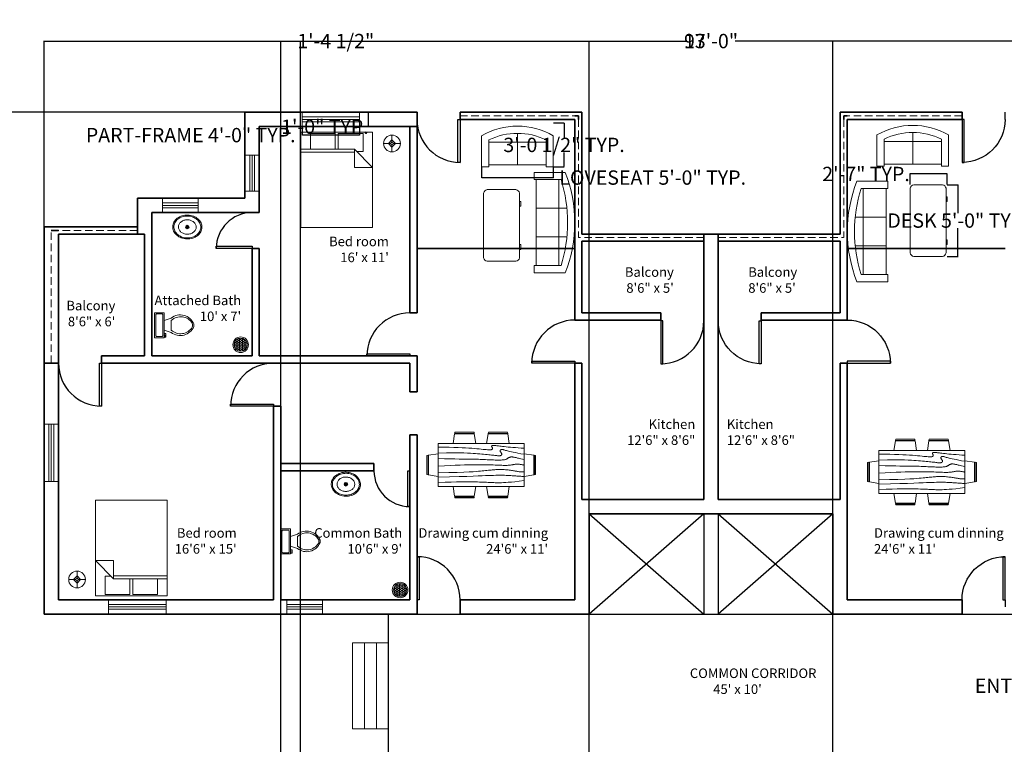
# Model space of a CAD drawing. Units: inches. Extents: x 2450 to 4494, y 1482 to 2597.
# Tile 6 of 7: x 3238 to 4062, y 1990 to 2597. Entities that reach past the tile are written whole.
import ezdxf

# ---------------------------------------------------------------- set-up
doc = ezdxf.new("R2010")
doc.units = ezdxf.units.IN
doc.header["$LTSCALE"] = 5
doc.header["$MEASUREMENT"] = 0
doc.linetypes.add('HIDDEN', pattern=[0.375, 0.25, -0.125])
for name, color, linetype, lineweight in [('A-ANNO-DIMS', 2, 'Continuous', 18), ('A-AREA-IDEN', 7, 'Continuous', 18), ('A-DOOR', 4, 'Continuous', 25), ('A-FLOR-EDGE', 7, 'Continuous', 25), ('A-FLOR-EVTR', 6, 'Continuous', 25), ('A-FLOR-FIXT', 9, 'Continuous', 18), ('A-FLOR-STRS', 7, 'Continuous', 18), ('A-FURN', 8, 'Continuous', 18), ('A-GLAZ', 4, 'Continuous', 18), ('A-WALL', 7, 'Continuous', 35), ('A-WALL-HIDN', 7, 'HIDDEN', 18)]:
    doc.layers.add(name, color=color, linetype=linetype, lineweight=lineweight)
doc.styles.get("Standard").update_dxf_attribs({"font": 'arial.ttf'})
doc.dimstyles.get("Standard").update_dxf_attribs({"dimtxt": 12, "dimasz": 0.18, "dimexe": 0.18, "dimexo": 0.0625, "dimgap": 0.09, "dimtad": 0, "dimtih": 1, "dimtoh": 1, "dimdec": 0, "dimzin": 0, "dimdsep": 46, "dimlunit": 3, "dimtxsty": 'Standard', "dimcen": 0.09, "dimadec": 0, "dimazin": 0, "dimtfac": 1, "dimtdec": 0, "dimtofl": 0, "dimtmove": 0, "dimatfit": 3, "dimfxl": 1, "dimtolj": 1, "dimtzin": 0, "dimarcsym": 0})

# ---------------------------------------------------------------- blocks, each defined once
blk = doc.blocks.new('*U4')
for p, q in [((-36, 0), (-36, -6)), ((0, 0), (0, -6))]:
    blk.add_line(p, q)
blk.add_lwpolyline([(0, 0), (0, 36), (-1.75, 36), (-1.75, 0)], close=True)
blk.add_arc((0, 0), 36, 90, 180)
blk = doc.blocks.new('*U2')
for p, q in [((0, 0), (0, -6)), ((36, 0), (36, -6))]:
    blk.add_line(p, q)
blk.add_lwpolyline([(0, 0), (0, 36), (1.75, 36), (1.75, 0)], close=True)
blk.add_arc((0, 0), 36, 0, 90)
blk = doc.blocks.new('*U5')
for p, q in [((-36, 0), (-36, 6)), ((0, 0), (0, 6))]:
    blk.add_line(p, q)
blk.add_lwpolyline([(0, 0), (0, -36), (-1.75, -36), (-1.75, 0)], close=True)
blk.add_arc((0, 0), 36, 180, 270)
blk = doc.blocks.new('*U3')
for p, q in [((0, 0), (0, -6)), ((30, 0), (30, -6))]:
    blk.add_line(p, q)
blk.add_lwpolyline([(0, 0), (0, 30), (1.75, 30), (1.75, 0)], close=True)
blk.add_arc((0, 0), 30, 0, 90)
blk = doc.blocks.new('Bed - Queen')
for p, q in [((0, -80.00003), (0, 0)), ((0, 0), (59.99999, 0)), ((59.99999, 0), (59.99999, -80.00003)), ((7.99999, -1.2), (28.79998, -1.2)), ((7.99999, -14.4), (7.99999, -1.2)), ((28.79998, -1.2), (28.79998, -14.4)), ((31.19999, -1.2), (51.99999, -1.2)), ((31.19999, -14.4), (31.19999, -1.2)), ((51.99999, -1.2), (51.99999, -16.4)), ((0, -14.4), (44.8, -14.4)), ((59.99999, -29.6), (44.8, -14.4)), ((44.8, -14.4), (44.8, -29.6)), ((51.99999, -16.4), (46.79936, -16.4)), ((44.8, -16.8), (0, -16.8)), ((44.8, -29.6), (59.99999, -29.6)), ((59.99999, -80.00003), (0, -80.00003))]:
    blk.add_line(p, q)
blk = doc.blocks.new('Lamp - Table')
for p, q in [((-1, 0), (-7, 0)), ((0, 3), (-3, 0)), ((-3, 0), (0, -3)), ((0, 7), (0, 1)), ((3, 0), (0, 3)), ((0, -3), (3, 0)), ((1, 0), (7, 0)), ((0, -1), (0, -7))]:
    blk.add_line(p, q)
for radius in [7, 1]:
    blk.add_circle((0, 0), radius)
blk = doc.blocks.new('Toilet - top')
for p, q in [((-8, -8.5), (-8, -8)), ((-7, -8), (-7, -9.5)), ((-4, -8), (-6, -14)), ((4, -8), (6, -14)), ((9.5, -6), (9.5, -2)), ((-10, -8.5), (-8, -8.5)), ((-10, -9.5), (-10, -8.5)), ((-7, -9.5), (-10, -9.5)), ((4, -14), (-4, -14))]:
    blk.add_line(p, q)
blk.add_lwpolyline([(10.5, -8), (10.5, 0), (-10.5, 0), (-10.5, -8)], close=True)
for points in [[(-9.5, -2), (-9.5, -6)], [(8.5, -1), (-8.5, -1)], [(-8.5, -7), (8.5, -7)]]:
    blk.add_lwpolyline(points)
for centre, radius, start, end in [((-8.62, -1.88), 0.884, 81.8699, 188.1301), ((-8.62, -6.12), 0.884, 171.8699, 278.1301), ((8.62, -1.88), 0.884, 351.8699, 98.1301), ((8.62, -6.12), 0.884, 261.8699, 8.1301), ((3.52, -21.58), 12.17, 141.46911, 247.97143), ((4.2, -21.82), 11.33, 136.36773, 238.94682), ((-3.52, -21.58), 12.17, 292.02843, 38.53071), ((-4.2, -21.82), 11.33, 301.05301, 43.63209), ((0, -27.88), 4, 245.73182, 294.26817), ((0, -29), 4, 254.86053, 285.13947)]:
    blk.add_arc(centre, radius, start, end)
blk = doc.blocks.new('Sink - Oval top')
for p, q in [((-1, 0), (1, 0)), ((0, 1), (0, -1))]:
    blk.add_line(p, q)
for points in [[(-12.23, 0.39, 0.117634), (-11.46, -3.36, 0.104469), (-8.88, -6.8, 0.090016), (-5.08, -9.07, 0.08192), (-0.32, -10.02, 0.08192), (4.49, -9.38, 0.090016), (8.42, -7.36, 0.104469), (11.22, -4.09, 0.117634), (12.23, -0.39, 0.117634), (11.46, 3.36, 0.104469), (8.88, 6.8, 0.090016), (5.08, 9.07, 0.08192), (0.32, 10.02, 0.08192), (-4.49, 9.38, 0.090016), (-8.42, 7.36, 0.104469), (-11.22, 4.09, 0.117634)], [(-11.29, 0.16, 0.118622), (-10.52, -3.25, 0.104678), (-8.07, -6.36, 0.089562), (-4.54, -8.37, 0.081185), (-0.13, -9.15, 0.081185), (4.3, -8.49, 0.089562), (7.89, -6.58, 0.104678), (10.42, -3.55, 0.118622), (11.29, -0.16, 0.118622), (10.52, 3.25, 0.104678), (8.07, 6.36, 0.089562), (4.54, 8.37, 0.081185), (0.13, 9.15, 0.081185), (-4.3, 8.49, 0.089562), (-7.89, 6.58, 0.104678), (-10.42, 3.55, 0.118622)], [(-7.42, 0.08, 0.118283), (-6.91, -2.17, 0.104607), (-5.29, -4.21, 0.089718), (-2.97, -5.53, 0.081436), (-0.07, -6.04, 0.081436), (2.84, -5.59, 0.089718), (5.2, -4.33, 0.104607), (6.86, -2.32, 0.118283), (7.42, -0.08, 0.118283), (6.91, 2.17, 0.104607), (5.29, 4.21, 0.089718), (2.97, 5.53, 0.081436), (0.07, 6.04, 0.081436), (-2.84, 5.59, 0.089718), (-5.2, 4.33, 0.104607), (-6.86, 2.32, 0.118283)]]:
    blk.add_lwpolyline(points, format="xyb", close=True)
for radius in [1.5, 1]:
    blk.add_circle((0, 0), radius)
blk = doc.blocks.new('Dining Set - 36 x 72 in.')
for p, q in [((-22.2343, 26.00059), (-23.4847, 17.99762)), ((-22.2304, 26), (-5.7608, 26)), ((-22, 27.5), (-22.1562, 26.50042)), ((-5.8416, 26.5), (-22.1534, 26.5)), ((-22, 27.5), (-6, 27.5)), ((-5.8437, 26.49966), (-6, 27.5)), ((-4.5152, 17.99762), (-5.7655, 25.99926)), ((5.7657, 26.00059), (4.5153, 17.99762)), ((5.7696, 26), (22.2392, 26)), ((6, 27.5), (5.8438, 26.50042)), ((22.1584, 26.5), (5.8466, 26.5)), ((6, 27.5), (22, 27.5)), ((22.1563, 26.49966), (22, 27.5)), ((23.4848, 17.99762), (22.2345, 25.99926)), ((36, 18), (-36, 18)), ((-36, 18), (-36, -18)), ((36, -18), (36, 18)), ((-44.0006, 8.23428), (-35.9976, 9.48474)), ((44.0006, 8.23428), (35.9976, 9.48474)), ((-45.5, 8), (-44.5004, 8.15617)), ((-45.5, 8), (-45.5, -8)), ((-44.5, -8.15843), (-44.5, 8.15338)), ((-44, 8.23041), (-44, -8.23915)), ((44, 8.23041), (44, -8.23915)), ((44.5, -8.15843), (44.5, 8.15338)), ((45.5, 8), (44.5005, 8.15617)), ((45.5, 8), (45.5, -8)), ((-44.4997, -8.15631), (-45.5, -8)), ((-35.9976, -9.48476), (-43.9993, -8.2345)), ((35.9976, -9.48476), (43.9993, -8.2345)), ((44.4997, -8.15631), (45.5, -8)), ((-36, -18), (36, -18)), ((-22.2343, -26.0006), (-23.4847, -17.99762)), ((-4.5152, -17.99762), (-5.7655, -25.99928)), ((5.7657, -26.0006), (4.5153, -17.99762)), ((23.4848, -17.99762), (22.2345, -25.99928)), ((-22.2304, -26), (-5.7608, -26)), ((-22, -27.5), (-22.1562, -26.50044)), ((-5.8416, -26.5), (-22.1534, -26.5)), ((-22, -27.5), (-6, -27.5)), ((-5.8437, -26.49967), (-6, -27.5)), ((5.7696, -26), (22.2392, -26)), ((6, -27.5), (5.8438, -26.50044)), ((22.1584, -26.5), (5.8466, -26.5)), ((6, -27.5), (22, -27.5)), ((22.1563, -26.49967), (22, -27.5))]:
    blk.add_line(p, q)
for points in [[(-36, 15), (-31.1772, 14.97754), (-26.8079, 14.91406), (-22.8538, 14.81543), (-19.276, 14.6875), (-16.0362, 14.53613), (-13.0957, 14.36718), (-10.4159, 14.18652), (-7.9583, 14), (-5.6904, 13.81315), (-3.6035, 13.63021), (-1.6954, 13.45508), (0.0365, 13.29166), (1.5945, 13.14388), (2.9811, 13.01562), (4.1988, 12.9108), (5.25, 12.83333), (6.1393, 12.78613), (6.8802, 12.76823), (7.4883, 12.77767), (7.9792, 12.8125), (8.3685, 12.87077), (8.6719, 12.95052), (8.9049, 13.0498), (9.0833, 13.16666), (9.2205, 13.29899), (9.3216, 13.44401), (9.3895, 13.59879), (9.4271, 13.76041), (9.4373, 13.92594), (9.4232, 14.09245), (9.3875, 14.257), (9.3333, 14.41666), (9.2638, 14.56917), (9.1836, 14.71484), (9.0975, 14.85465), (9.0104, 14.98958), (8.9272, 15.1206), (8.8529, 15.2487), (8.7922, 15.37483), (8.75, 15.5), (8.7305, 15.62467), (8.7344, 15.74739), (8.7617, 15.86621), (8.8125, 15.97916), (8.8867, 16.08431), (8.9844, 16.17968), (9.1055, 16.26334), (9.25, 16.33333), (9.4189, 16.38802), (9.6172, 16.42708), (9.8506, 16.45052), (10.125, 16.45833), (10.4463, 16.45052), (10.8203, 16.42708), (11.2529, 16.38802), (11.75, 16.33333), (12.3184, 16.26318), (12.9694, 16.17838), (13.7151, 16.07991), (14.5677, 15.96875), (15.5395, 15.84586), (16.6426, 15.71224), (17.8893, 15.56884), (19.2917, 15.41666), (20.859, 15.25667), (22.5879, 15.08984), (24.4721, 14.91715), (26.5052, 14.73958), (28.6809, 14.5581), (30.9929, 14.3737), (33.4347, 14.18733), (36, 14)], [(-36, 10), (-28.9766, 10.14274), (-23.1725, 10.20442), (-18.4241, 10.19775), (-14.5677, 10.13541), (-11.4399, 10.03011), (-8.877, 9.89453), (-6.7154, 9.74137), (-4.7917, 9.58333), (-2.9698, 9.43082), (-1.2246, 9.28515), (0.4415, 9.14534), (2.026, 9.01041), (3.5266, 8.87939), (4.9408, 8.7513), (6.266, 8.62516), (7.5, 8.5), (8.6411, 8.37549), (9.6914, 8.2539), (10.6538, 8.13818), (11.5312, 8.03125), (12.3267, 7.93603), (13.043, 7.85547), (13.6831, 7.79248), (14.25, 7.75), (14.7471, 7.7303), (15.1797, 7.73307), (15.5537, 7.75732), (15.875, 7.80208), (16.1494, 7.86637), (16.3828, 7.94922), (16.5811, 8.04964), (16.75, 8.16666), (16.8944, 8.29915), (17.0143, 8.44531), (17.1089, 8.60319), (17.1771, 8.77083), (17.218, 8.94629), (17.2305, 9.1276), (17.2137, 9.31282), (17.1667, 9.5), (17.0895, 9.6875), (16.987, 9.875), (16.8649, 10.0625), (16.7292, 10.25), (16.5856, 10.4375), (16.4401, 10.625), (16.2985, 10.8125), (16.1667, 11), (16.05, 11.18733), (15.9518, 11.3737), (15.8752, 11.5581), (15.8229, 11.73958), (15.798, 11.91715), (15.8034, 12.08984), (15.842, 12.25667), (15.9167, 12.41666), (16.0295, 12.56836), (16.1784, 12.70833), (16.3605, 12.83268), (16.5729, 12.9375), (16.8127, 13.01888), (17.0768, 13.07291), (17.3625, 13.0957), (17.6667, 13.08333), (17.9894, 13.03312), (18.3418, 12.94726), (18.7382, 12.82918), (19.1927, 12.68229), (19.7195, 12.51001), (20.3327, 12.31575), (21.0465, 12.10294), (21.875, 11.875), (22.8357, 11.63354), (23.959, 11.37304), (25.2786, 11.08618), (26.8282, 10.76562), (28.6414, 10.40405), (30.752, 9.99414), (33.1936, 9.52856), (36, 9)], [(-36, 5.5), (-30.7157, 5.3348), (-26.069, 5.20963), (-21.9946, 5.11767), (-18.4271, 5.05208), (-15.3009, 5.00602), (-12.5508, 4.97265), (-10.1112, 4.94515), (-7.9167, 4.91666), (-5.909, 4.88167), (-4.0586, 4.83984), (-2.3429, 4.79215), (-0.7396, 4.73958), (0.7739, 4.6831), (2.22, 4.6237), (3.6213, 4.56233), (5, 4.5), (6.373, 4.43782), (7.7344, 4.3776), (9.0723, 4.32129), (10.375, 4.27083), (11.6309, 4.22819), (12.8281, 4.19531), (13.9551, 4.17415), (15, 4.16666), (15.954, 4.17448), (16.819, 4.19791), (17.6001, 4.23698), (18.3021, 4.29166), (18.9299, 4.36198), (19.4883, 4.44791), (19.9823, 4.54948), (20.4167, 4.66666), (20.7969, 4.79899), (21.1302, 4.94401), (21.4245, 5.09879), (21.6875, 5.26041), (21.9271, 5.42594), (22.1511, 5.59245), (22.3672, 5.757), (22.5834, 5.91666), (22.8065, 6.06868), (23.0404, 6.21093), (23.2879, 6.34147), (23.5521, 6.45833), (23.8358, 6.55957), (24.142, 6.64323), (24.4735, 6.70735), (24.8334, 6.75), (25.2235, 6.76969), (25.642, 6.76692), (26.0858, 6.74267), (26.5521, 6.69791), (27.0379, 6.63362), (27.5404, 6.55078), (28.0565, 6.45036), (28.5834, 6.33333), (29.1242, 6.19987), (29.7071, 6.04687), (30.3661, 5.87044), (31.1354, 5.66666), (32.0493, 5.43164), (33.142, 5.16146), (34.4475, 4.85221), (36, 4.5)], [(-36, -1), (-30.7915, -0.6591), (-26.0195, -0.38216), (-21.6519, -0.16284), (-17.6563, 0.00521), (-14.0005, 0.12833), (-10.6523, 0.21289), (-7.5796, 0.26522), (-4.75, 0.29166), (-2.134, 0.29793), (0.2878, 0.28711), (2.5317, 0.26163), (4.6146, 0.22396), (6.5529, 0.17651), (8.3633, 0.12174), (10.0623, 0.06209), (11.6667, 0), (13.1899, -0.06201), (14.6341, -0.1211), (15.9982, -0.17432), (17.2813, -0.21875), (18.4823, -0.25147), (19.6003, -0.26953), (20.6343, -0.27002), (21.5834, -0.25), (22.4481, -0.20768), (23.2357, -0.14584), (23.9549, -0.06836), (24.6146, 0.02083), (25.2235, 0.11784), (25.7904, 0.21875), (26.3241, 0.31966), (26.8334, 0.41666), (27.3265, 0.50618), (27.8099, 0.58593), (28.2894, 0.65397), (28.7709, 0.70833), (29.2601, 0.74707), (29.763, 0.76823), (30.2855, 0.76985), (30.8334, 0.75), (31.4088, 0.70784), (31.9994, 0.64713), (32.589, 0.57275), (33.1615, 0.48958), (33.7008, 0.4025), (34.1908, 0.3164), (34.6153, 0.23616), (34.9584, 0.16666), (35.2099, 0.11165), (35.3848, 0.07031), (35.504, 0.04069), (35.5886, 0.02083), (35.6594, 0.00879), (35.7377, 0.0026), (35.8442, 0.00032), (36, 0)], [(-36, -6.5), (-27.1843, -6.31267), (-20.084, -6.1263), (-14.469, -5.9419), (-10.1094, -5.76042), (-6.7752, -5.58285), (-4.2363, -5.41016), (-2.2629, -5.24333), (-0.625, -5.08334), (0.8708, -4.93099), (2.2715, -4.78646), (3.5872, -4.64974), (4.8281, -4.52084), (6.0046, -4.39974), (7.127, -4.28646), (8.2053, -4.18099), (9.25, -4.08334), (10.2705, -3.99382), (11.2734, -3.91407), (12.2647, -3.84603), (13.25, -3.79167), (14.2354, -3.75293), (15.2266, -3.73177), (16.2295, -3.73015), (17.25, -3.75), (18.2912, -3.79248), (19.3451, -3.85547), (20.4009, -3.93604), (21.4479, -4.03125), (22.4754, -4.13819), (23.4727, -4.25391), (24.4289, -4.37549), (25.3334, -4.5), (26.1785, -4.62492), (26.9694, -4.74935), (27.7145, -4.87281), (28.4219, -4.99479), (29.1, -5.11483), (29.7572, -5.23242), (30.4016, -5.34709), (31.0417, -5.45834), (31.6837, -5.56437), (32.3262, -5.65821), (32.9658, -5.73153), (33.599, -5.77604), (34.2224, -5.78345), (34.8327, -5.74545), (35.4264, -5.65373), (36, -5.5)], [(-36, -10), (-26.4022, -9.81299), (-18.4675, -9.62891), (-11.9839, -9.45069), (-6.7396, -9.28125), (-2.5226, -9.12354), (0.8789, -8.98047), (3.6769, -8.85498), (6.0833, -8.75), (8.2767, -8.66765), (10.3021, -8.60677), (12.1712, -8.56543), (13.8958, -8.54167), (15.4876, -8.53353), (16.9583, -8.53907), (18.3197, -8.55632), (19.5834, -8.58334), (20.7616, -8.61841), (21.8685, -8.66081), (22.9188, -8.71004), (23.9271, -8.76563), (24.9081, -8.82707), (25.8763, -8.89388), (26.8465, -8.96558), (27.8334, -9.04167), (28.8474, -9.12118), (29.8828, -9.20117), (30.93, -9.27824), (31.9792, -9.34896), (33.0205, -9.40991), (34.0443, -9.45768), (35.0407, -9.48885), (36, -9.5)], [(-36, -14.5), (-30.0881, -14.33513), (-25.0332, -14.21224), (-20.7312, -14.12647), (-17.0781, -14.07292), (-13.97, -14.04671), (-11.3027, -14.04297), (-8.9724, -14.05681), (-6.875, -14.08334), (-4.9224, -14.11833), (-3.0905, -14.16016), (-1.3709, -14.20785), (0.2448, -14.26042), (1.7647, -14.3169), (3.1973, -14.3763), (4.5507, -14.43767), (5.8333, -14.5), (7.0554, -14.5621), (8.235, -14.62175), (9.3922, -14.67652), (10.5469, -14.72396), (11.7192, -14.76164), (12.929, -14.78711), (14.1965, -14.79794), (15.5417, -14.79167), (16.9933, -14.76424), (18.6152, -14.70508), (20.4804, -14.60197), (22.6615, -14.44271), (25.2312, -14.21509), (28.2624, -13.9069), (31.8277, -13.50594), (36, -13)]]:
    blk.add_lwpolyline(points)
blk = doc.blocks.new('Sofa - Roundback Loveseat 5 ft.')
for p, q in [((0, -32.44198), (0, -5.99998)), ((-24, -33.99998), (-24, -11.46958)), ((-23.9998, -13.38178), (23.99986, -13.38178)), ((24.00004, -33.99998), (24.00004, -11.46958)), ((-24, -32.44198), (24.00004, -32.44198))]:
    blk.add_line(p, q)
for points in [[(-24, -33.99998), (-30, -33.99998), (-30, -7.99998)], [(30.00004, -7.99998), (30.00004, -33.99998), (24.00004, -33.99998)]]:
    blk.add_lwpolyline(points)
for centre, radius, start, end in [((0, -60.24998), 60.24998, 60.13715, 119.8628), ((0, -61.38438), 55.38444, 64.32083, 115.6792)]:
    blk.add_arc(centre, radius, start, end)
blk = doc.blocks.new('Sofa - Roundback 7 ft.')
for p, q in [((-12.00002, -32.4421), (-12.00003, -6.5971)), ((11.99997, -32.4421), (11.99998, -6.5971)), ((-36.000027, -34), (-36.000027, -11.4696)), ((-35.999844, -13.3819), (35.9998, -13.3819)), ((35.99998, -34), (35.99998, -11.4696)), ((-36.000027, -32.4421), (35.99998, -32.4421))]:
    blk.add_line(p, q)
for points in [[(-36.000027, -34), (-42.000027, -34), (-42.000027, -8)], [(41.99998, -8), (41.99998, -34), (35.99998, -34)]]:
    blk.add_lwpolyline(points)
for centre, radius, start, end in [((0, -114.25), 114.25, 68.43141, 111.5686), ((-0.00001, -127.1968), 121.1968, 72.72033, 107.2797)]:
    blk.add_arc(centre, radius, start, end)
blk = doc.blocks.new('Desk - 30 x 60 in.')
for p, q in [((-26.999995, 0), (26.999995, 0)), ((-29.999995, -27), (-29.999995, -3)), ((29.999995, -3), (29.999995, -27)), ((26.999995, -30), (-26.999995, -30)), ((-20.000005, -30), (-20.000005, -31)), ((-20.000005, -31), (-16.000005, -31)), ((-16.000005, -31), (-16.000005, -30)), ((15.999995, -31), (15.999995, -30)), ((19.999995, -31), (15.999995, -31)), ((19.999995, -30), (19.999995, -31))]:
    blk.add_line(p, q)
for centre, start, end in [((-26.499995, -3.5), 98.1301, 171.8699), ((26.499995, -3.5), 8.130102, 81.8699), ((-26.499995, -26.5), 188.1301, 261.8699), ((26.499995, -26.5), 278.1301, 351.8699)]:
    blk.add_arc(centre, 3.535534, start, end)
blk = doc.blocks.new('WIN-30-FRAME')
for p, q in [((0, 0), (0, 12)), ((0, 12), (30, 12)), ((30, 12), (30, 0)), ((30, 8), (0, 8)), ((30, 6), (0, 6)), ((30, 4), (0, 4)), ((30, 0), (0, 0))]:
    blk.add_line(p, q)
blk = doc.blocks.new('WIN-48-FRAME')
for p, q in [((48, 12), (0, 12)), ((0, 12), (0, 0)), ((48, 0), (48, 12)), ((48, 8), (0, 8)), ((48, 6), (0, 6)), ((48, 4), (0, 4)), ((0, 0), (48, 0))]:
    blk.add_line(p, q)
blk = doc.blocks.new('WIN-30-PART-FRAME')
for p, q in [((12, 30), (0, 30)), ((0, 30), (0, 0)), ((4, 30), (4, 0)), ((6, 30), (6, 0)), ((8, 30), (8, 0)), ((12, 6), (12, 30)), ((0, 0), (12, 0))]:
    blk.add_line(p, q)
blk = doc.blocks.new('WIN-48-PART-FRAME')
for p, q in [((48, 12), (0, 12)), ((0, 12), (0, 0)), ((48, 0), (48, 12)), ((48, 8), (0, 8)), ((48, 6), (0, 6)), ((48, 4), (0, 4)), ((24, 0), (48, 0))]:
    blk.add_line(p, q)
blk = doc.blocks.new('WIN-48-OPEN-SIDE')
for p, q in [((0, 48), (12, 48)), ((4, 48), (4, 0)), ((6, 48), (6, 0)), ((8, 48), (8, 0)), ((12, 48), (12, 0)), ((12, 0), (0, 0))]:
    blk.add_line(p, q)
blk = doc.blocks.new('STEPS-72-ENTRY')
at = {"ltscale": 5}
for p, q in [((0, 72), (30, 72)), ((10, 0), (10, 72)), ((20, 0), (20, 72)), ((30, 0), (30, 72)), ((0, 0), (30, 0))]:
    blk.add_line(p, q, dxfattribs=at)
blk = doc.blocks.new('DRAIN-FLOOR-ROUND')
at = {"ltscale": 5}
h = blk.add_hatch(dxfattribs=at)
h.set_pattern_fill('HONEY', color=256, scale=7)
h.set_pattern_definition([(0, (-4161.689, -1861.538), (1.3125, 0.75777223), [0.875, -1.75]), (120, (-4161.689, -1861.538), (-1.3125, 0.75777223), [0.875, -1.75]), (60, (-4161.689, -1861.538), (3e-16, 1.51554446), [-1.75, 0.875])])
h.paths.add_polyline_path([(1, 6.52, 1), (12.03, 6.52, 1)])
for radius in [6.52, 5.52]:
    blk.add_circle((6.52, 6.52), radius, dxfattribs=at)
blk = doc.blocks.new('*D45')
at = {"layer": 'A-ANNO-DIMS', "color": 0, "lineweight": -2, "ltscale": 5, "transparency": 16777216}
for p, q in [((3474.29, 2507.2), (3474.29, 2499.89)), ((3522.29, 2507.2), (3522.29, 2499.89)), ((3474.29, 2500.07), (3474.11, 2500.07)), ((3522.11, 2500.07), (3474.47, 2500.07))]:
    blk.add_line(p, q, dxfattribs=at)
at = {"layer": 'A-ANNO-DIMS', "color": 0, "ltscale": 5, "transparency": 16777216}
for points in [[(3474.47, 2500.1), (3474.47, 2500.04), (3474.29, 2500.07)], [(3522.11, 2500.1), (3522.11, 2500.04), (3522.29, 2500.07)]]:
    blk.add_solid(points, dxfattribs=at)
at = {"layer": 'Defpoints', "color": 0, "ltscale": 5, "transparency": 16777216}
for p in [(3474.29, 2507.27), (3522.29, 2507.27), (3474.29, 2500.07)]:
    blk.add_point(p, dxfattribs=at)
at = {"layer": 'A-ANNO-DIMS', "color": 0, "ltscale": 5, "transparency": 16777216, "insert": (3380.93, 2500.07), "char_height": 12, "attachment_point": 5}
blk.add_mtext('\\A1;PART-FRAME 4\'-0" TYP.', dxfattribs=at)
blk = doc.blocks.new('*D46')
at = {"layer": 'A-ANNO-DIMS', "color": 0, "lineweight": -2, "ltscale": 5, "transparency": 16777216}
for p, q in [((3522.35, 2519.27), (3529.67, 2519.27)), ((3529.49, 2519.09), (3529.49, 2507.45)), ((3522.35, 2507.27), (3529.67, 2507.27)), ((3529.49, 2507.09), (3529.31, 2507.09)), ((3529.49, 2507.27), (3529.49, 2507.09))]:
    blk.add_line(p, q, dxfattribs=at)
at = {"layer": 'A-ANNO-DIMS', "color": 0, "ltscale": 5, "transparency": 16777216}
for points in [[(3529.46, 2519.09), (3529.52, 2519.09), (3529.49, 2519.27)], [(3529.46, 2507.45), (3529.52, 2507.45), (3529.49, 2507.27)]]:
    blk.add_solid(points, dxfattribs=at)
at = {"layer": 'Defpoints', "color": 0, "ltscale": 5, "transparency": 16777216}
for p in [(3522.29, 2519.27), (3522.29, 2507.27), (3529.49, 2507.27)]:
    blk.add_point(p, dxfattribs=at)
at = {"layer": 'A-ANNO-DIMS', "color": 0, "ltscale": 5, "transparency": 16777216, "insert": (3493.21, 2507.09), "char_height": 12, "attachment_point": 5}
blk.add_mtext('\\A1;1\'-0" TYP.', dxfattribs=at)
blk = doc.blocks.new('*D61')
at = {"layer": 'A-ANNO-DIMS', "color": 0, "lineweight": -2, "ltscale": 5, "transparency": 16777216}
for p, q in [((3624.29, 2473.48), (3624.29, 2464.37)), ((3684.29, 2473.48), (3684.29, 2464.37)), ((3624.47, 2464.55), (3684.11, 2464.55)), ((3684.29, 2464.55), (3684.47, 2464.55))]:
    blk.add_line(p, q, dxfattribs=at)
at = {"layer": 'A-ANNO-DIMS', "color": 0, "ltscale": 5, "transparency": 16777216}
for points in [[(3624.47, 2464.58), (3624.47, 2464.52), (3624.29, 2464.55)], [(3684.11, 2464.58), (3684.11, 2464.52), (3684.29, 2464.55)]]:
    blk.add_solid(points, dxfattribs=at)
at = {"layer": 'Defpoints', "color": 0, "ltscale": 5, "transparency": 16777216}
for p in [(3624.29, 2473.55), (3684.29, 2473.55), (3684.29, 2464.55)]:
    blk.add_point(p, dxfattribs=at)
at = {"layer": 'A-ANNO-DIMS', "color": 0, "ltscale": 5, "transparency": 16777216, "insert": (3767.45, 2464.55), "char_height": 12, "attachment_point": 5}
blk.add_mtext('\\A1;LOVESEAT 5\'-0" TYP.', dxfattribs=at)
blk = doc.blocks.new('*D62')
at = {"layer": 'A-ANNO-DIMS', "color": 0, "lineweight": -2, "ltscale": 5, "transparency": 16777216}
for p, q in [((3684.35, 2510.21), (3693.47, 2510.21)), ((3693.29, 2510.03), (3693.29, 2498.18)), ((3693.29, 2473.73), (3693.29, 2485.58)), ((3684.35, 2473.55), (3693.47, 2473.55))]:
    blk.add_line(p, q, dxfattribs=at)
at = {"layer": 'A-ANNO-DIMS', "color": 0, "ltscale": 5, "transparency": 16777216}
for points in [[(3693.26, 2510.03), (3693.32, 2510.03), (3693.29, 2510.21)], [(3693.26, 2473.73), (3693.32, 2473.73), (3693.29, 2473.55)]]:
    blk.add_solid(points, dxfattribs=at)
at = {"layer": 'Defpoints', "color": 0, "ltscale": 5, "transparency": 16777216}
for p in [(3684.29, 2510.21), (3693.29, 2510.21), (3684.29, 2473.55)]:
    blk.add_point(p, dxfattribs=at)
at = {"layer": 'A-ANNO-DIMS', "color": 0, "ltscale": 5, "transparency": 16777216, "insert": (3693.29, 2491.88), "char_height": 12, "attachment_point": 5}
blk.add_mtext('\\A1;3\'-0 1/2" TYP.', dxfattribs=at)
blk = doc.blocks.new('*D65')
at = {"layer": 'A-ANNO-DIMS', "color": 0, "lineweight": -2, "ltscale": 5, "transparency": 16777216}
for p, q in [((4013.95, 2458.56), (4023.07, 2458.56)), ((4022.89, 2458.38), (4022.89, 2434.86)), ((4022.89, 2398.74), (4022.89, 2422.27)), ((4013.95, 2398.56), (4023.07, 2398.56))]:
    blk.add_line(p, q, dxfattribs=at)
at = {"layer": 'A-ANNO-DIMS', "color": 0, "ltscale": 5, "transparency": 16777216}
for points in [[(4022.86, 2458.38), (4022.92, 2458.38), (4022.89, 2458.56)], [(4022.86, 2398.74), (4022.92, 2398.74), (4022.89, 2398.56)]]:
    blk.add_solid(points, dxfattribs=at)
at = {"layer": 'Defpoints', "color": 0, "ltscale": 5, "transparency": 16777216}
for p in [(4013.89, 2458.56), (4022.89, 2458.56), (4013.89, 2398.56)]:
    blk.add_point(p, dxfattribs=at)
at = {"layer": 'A-ANNO-DIMS', "color": 0, "ltscale": 5, "transparency": 16777216, "insert": (4022.89, 2428.56), "char_height": 12, "attachment_point": 5}
blk.add_mtext('\\A1;DESK 5\'-0" TYP.', dxfattribs=at)
blk = doc.blocks.new('*D66')
at = {"layer": 'A-ANNO-DIMS', "color": 0, "lineweight": -2, "ltscale": 5, "transparency": 16777216}
for p, q in [((3982.89, 2467.56), (3982.71, 2467.56)), ((3982.89, 2458.62), (3982.89, 2467.74)), ((4013.71, 2467.56), (3983.07, 2467.56)), ((4013.89, 2458.62), (4013.89, 2467.74))]:
    blk.add_line(p, q, dxfattribs=at)
at = {"layer": 'A-ANNO-DIMS', "color": 0, "ltscale": 5, "transparency": 16777216}
for points in [[(3983.07, 2467.59), (3983.07, 2467.53), (3982.89, 2467.56)], [(4013.71, 2467.59), (4013.71, 2467.53), (4013.89, 2467.56)]]:
    blk.add_solid(points, dxfattribs=at)
at = {"layer": 'Defpoints', "color": 0, "ltscale": 5, "transparency": 16777216}
for p in [(3982.89, 2467.56), (3982.89, 2458.56), (4013.89, 2458.56)]:
    blk.add_point(p, dxfattribs=at)
at = {"layer": 'A-ANNO-DIMS', "color": 0, "ltscale": 5, "transparency": 16777216, "insert": (3945.94, 2467.56), "char_height": 12, "attachment_point": 5}
blk.add_mtext('\\A1;2\'-7" TYP.', dxfattribs=at)
blk = doc.blocks.new('*D67')
at = {"layer": 'A-ANNO-DIMS', "color": 0, "lineweight": -2, "ltscale": 5, "transparency": 16777216}
for p, q in [((4116.35, 2075.27), (4127.27, 2075.27)), ((4127.09, 2075.09), (4127.09, 2045.56)), ((4127.09, 2003.45), (4127.09, 2032.97)), ((4116.35, 2003.27), (4127.27, 2003.27))]:
    blk.add_line(p, q, dxfattribs=at)
at = {"layer": 'A-ANNO-DIMS', "color": 0, "ltscale": 5, "transparency": 16777216}
for points in [[(4127.06, 2075.09), (4127.12, 2075.09), (4127.09, 2075.27)], [(4127.06, 2003.45), (4127.12, 2003.45), (4127.09, 2003.27)]]:
    blk.add_solid(points, dxfattribs=at)
at = {"layer": 'Defpoints', "color": 0, "ltscale": 5, "transparency": 16777216}
for p in [(4116.29, 2075.27), (4127.09, 2075.27), (4116.29, 2003.27)]:
    blk.add_point(p, dxfattribs=at)
at = {"layer": 'A-ANNO-DIMS', "color": 0, "ltscale": 5, "transparency": 16777216, "insert": (4127.09, 2039.27), "char_height": 12, "attachment_point": 5}
blk.add_mtext('\\A1;ENTRY STEPS 6\'-0" TYP.', dxfattribs=at)
blk = doc.blocks.new('*D71')
at = {"layer": 'A-ANNO-DIMS', "color": 0, "lineweight": -2, "ltscale": 5, "transparency": 16777216}
for p, q in [((3258.29, 2423.33), (3258.29, 2578.95)), ((3258.47, 2578.77), (3795.59, 2578.77)), ((4374.11, 2578.77), (3836.99, 2578.77)), ((4374.29, 2423.33), (4374.29, 2578.95))]:
    blk.add_line(p, q, dxfattribs=at)
at = {"layer": 'A-ANNO-DIMS', "color": 0, "ltscale": 5, "transparency": 16777216}
for points in [[(3258.47, 2578.8), (3258.47, 2578.74), (3258.29, 2578.77)], [(4374.11, 2578.8), (4374.11, 2578.74), (4374.29, 2578.77)]]:
    blk.add_solid(points, dxfattribs=at)
at = {"layer": 'Defpoints', "color": 0, "ltscale": 5, "transparency": 16777216}
for p in [(4374.29, 2578.77), (3258.29, 2423.27), (4374.29, 2423.27)]:
    blk.add_point(p, dxfattribs=at)
at = {"layer": 'A-ANNO-DIMS', "color": 0, "ltscale": 5, "transparency": 16777216, "insert": (3816.29, 2578.77), "char_height": 12, "attachment_point": 5}
blk.add_mtext('\\A1;93\'-0"', dxfattribs=at)
blk = doc.blocks.new('*D72')
at = {"layer": 'A-ANNO-DIMS', "color": 0, "lineweight": -2, "ltscale": 5, "transparency": 16777216}
for p, q in [((3426.23, 2519.27), (3198.61, 2519.27)), ((3198.79, 2519.09), (3198.79, 2045.48)), ((3198.79, 1559.45), (3198.79, 2033.05)), ((3426.23, 1559.27), (3198.61, 1559.27))]:
    blk.add_line(p, q, dxfattribs=at)
at = {"layer": 'A-ANNO-DIMS', "color": 0, "ltscale": 5, "transparency": 16777216}
for points in [[(3198.76, 2519.09), (3198.82, 2519.09), (3198.79, 2519.27)], [(3198.76, 1559.45), (3198.82, 1559.45), (3198.79, 1559.27)]]:
    blk.add_solid(points, dxfattribs=at)
at = {"layer": 'Defpoints', "color": 0, "ltscale": 5, "transparency": 16777216}
for p in [(3198.79, 2519.27), (3426.29, 2519.27), (3426.29, 1559.27)]:
    blk.add_point(p, dxfattribs=at)
at = {"layer": 'A-ANNO-DIMS', "color": 0, "ltscale": 5, "transparency": 16777216, "insert": (3198.79, 2039.27), "char_height": 12, "attachment_point": 5}
blk.add_mtext('\\A1;80\'-0"', dxfattribs=at)
blk = doc.blocks.new('*D73')
at = {"layer": 'A-ANNO-DIMS', "color": 0, "lineweight": -2, "ltscale": 5, "transparency": 16777216}
for p, q in [((3714.29, 1979.33), (3714.29, 2578.95)), ((3714.47, 2578.77), (3796.15, 2578.77)), ((3918.11, 2578.77), (3836.43, 2578.77)), ((3918.29, 1979.33), (3918.29, 2578.95))]:
    blk.add_line(p, q, dxfattribs=at)
at = {"layer": 'A-ANNO-DIMS', "color": 0, "ltscale": 5, "transparency": 16777216}
for points in [[(3714.47, 2578.8), (3714.47, 2578.74), (3714.29, 2578.77)], [(3918.11, 2578.8), (3918.11, 2578.74), (3918.29, 2578.77)]]:
    blk.add_solid(points, dxfattribs=at)
at = {"layer": 'Defpoints', "color": 0, "ltscale": 5, "transparency": 16777216}
for p in [(3918.29, 2578.77), (3714.29, 1979.27), (3918.29, 1979.27)]:
    blk.add_point(p, dxfattribs=at)
at = {"layer": 'A-ANNO-DIMS', "color": 0, "ltscale": 5, "transparency": 16777216, "insert": (3816.29, 2578.77), "char_height": 12, "attachment_point": 5}
blk.add_mtext('\\A1;17\'-0"', dxfattribs=at)
blk = doc.blocks.new('*D82')
at = {"layer": 'A-ANNO-DIMS', "color": 0, "lineweight": -2, "ltscale": 5, "transparency": 16777216}
for p, q in [((3456.29, 1967.33), (3456.29, 2578.95)), ((3456.47, 2578.77), (3472.48, 2578.77)), ((3472.66, 1967.33), (3472.66, 2578.95)), ((3472.66, 2578.77), (3472.84, 2578.77))]:
    blk.add_line(p, q, dxfattribs=at)
at = {"layer": 'A-ANNO-DIMS', "color": 0, "ltscale": 5, "transparency": 16777216}
for points in [[(3456.47, 2578.8), (3456.47, 2578.74), (3456.29, 2578.77)], [(3472.48, 2578.8), (3472.48, 2578.74), (3472.66, 2578.77)]]:
    blk.add_solid(points, dxfattribs=at)
at = {"layer": 'Defpoints', "color": 0, "ltscale": 5, "transparency": 16777216}
for p in [(3472.66, 2578.77), (3456.29, 1967.27), (3472.66, 1967.27)]:
    blk.add_point(p, dxfattribs=at)
at = {"layer": 'A-ANNO-DIMS', "color": 0, "ltscale": 5, "transparency": 16777216, "insert": (3502.3, 2578.77), "char_height": 12, "attachment_point": 5}
blk.add_mtext('\\A1;1\'-4 1/2"', dxfattribs=at)

msp = doc.modelspace()

# ---------------------------------------------------------------- linework, layer by layer
at = {"layer": 'A-FLOR-EDGE', "ltscale": 5}
for p, q in [((3546.29, 1979.27), (3546.29, 2099.27)), ((3546.29, 2099.27), (4086.29, 2099.27))]:
    msp.add_line(p, q, dxfattribs=at)
at = {"layer": 'A-FLOR-EVTR', "ltscale": 5}
for p, q in [((3810.29, 2183.27), (3714.29, 2099.27)), ((3714.29, 2183.27), (3810.29, 2099.27)), ((3810.29, 2183.27), (3810.29, 2099.27)), ((3822.29, 2183.27), (3822.29, 2099.27)), ((3822.29, 2183.27), (3918.29, 2099.27)), ((3918.29, 2183.27), (3822.29, 2099.27)), ((3714.29, 2099.27), (3918.29, 2099.27))]:
    msp.add_line(p, q, dxfattribs=at)
at = {"layer": 'A-WALL'}
for p, q in [((3570.29, 2519.27), (3426.29, 2519.27)), ((3426.29, 2507.27), (3426.29, 2519.27)), ((3570.29, 2507.27), (3570.29, 2519.27)), ((3708.29, 2519.27), (3606.29, 2519.27)), ((3606.29, 2513.27), (3606.29, 2519.27)), ((3702.29, 2513.27), (3606.29, 2513.27)), ((3702.29, 2516.27), (3705.29, 2516.27)), ((3702.29, 2345.27), (3702.29, 2513.27)), ((3705.29, 2513.27), (3705.29, 2516.27)), ((3708.29, 2507.27), (3708.29, 2519.27)), ((3924.29, 2519.27), (4026.29, 2519.27)), ((3924.29, 2507.27), (3924.29, 2519.27)), ((3927.29, 2513.27), (3927.29, 2516.27)), ((3930.29, 2516.27), (3927.29, 2516.27)), ((3930.29, 2513.27), (4026.29, 2513.27)), ((3930.29, 2345.27), (3930.29, 2513.27)), ((4026.29, 2513.27), (4026.29, 2519.27)), ((3426.29, 2507.27), (3426.29, 2447.27)), ((3570.29, 2507.27), (3438.29, 2507.27)), ((3438.29, 2507.27), (3438.29, 2435.27)), ((3564.29, 2351.27), (3564.29, 2507.27)), ((3570.29, 2351.27), (3570.29, 2507.27)), ((3708.29, 2417.27), (3708.29, 2507.27)), ((3924.29, 2417.27), (3924.29, 2507.27)), ((3336.29, 2447.27), (3336.29, 2423.27)), ((3348.29, 2447.27), (3336.29, 2447.27)), ((3348.29, 2447.27), (3426.29, 2447.27)), ((3348.29, 2435.27), (3348.29, 2315.27)), ((3348.29, 2435.27), (3432.29, 2435.27)), ((3432.29, 2435.27), (3438.29, 2435.27)), ((3258.29, 2423.27), (3258.29, 2099.27)), ((3270.29, 2423.27), (3258.29, 2423.27)), ((3270.29, 2423.27), (3336.29, 2423.27)), ((3336.29, 2423.27), (3336.29, 2417.27)), ((3270.29, 2420.27), (3264.29, 2420.27)), ((3270.29, 2417.27), (3270.29, 2315.27)), ((3270.29, 2417.27), (3342.29, 2417.27)), ((3342.29, 2417.27), (3342.29, 2315.27)), ((3708.29, 2417.27), (3810.29, 2417.27)), ((3822.29, 2417.27), (3810.29, 2417.27)), ((3810.29, 2417.27), (3822.29, 2417.27)), ((3810.29, 2411.27), (3810.29, 2417.27)), ((3822.29, 2195.27), (3822.29, 2417.27)), ((3924.29, 2417.27), (3822.29, 2417.27)), ((3822.29, 2411.27), (3822.29, 2417.27)), ((3822.29, 2195.27), (3822.29, 2417.27)), ((3708.29, 2411.27), (3810.29, 2411.27)), ((3708.29, 2351.27), (3708.29, 2411.27)), ((3810.29, 2351.27), (3810.29, 2411.27)), ((3924.29, 2411.27), (3822.29, 2411.27)), ((3822.29, 2351.27), (3822.29, 2411.27)), ((3924.29, 2351.27), (3924.29, 2411.27)), ((3432.29, 2405.27), (3432.29, 2315.27)), ((3432.29, 2405.27), (3438.29, 2405.27)), ((3438.29, 2405.27), (3438.29, 2315.27)), ((3570.29, 2405.27), (3702.29, 2405.27)), ((4062.29, 2405.27), (3930.29, 2405.27)), ((3564.29, 2351.27), (3570.29, 2351.27)), ((3708.29, 2351.27), (3774.29, 2351.27)), ((3774.29, 2345.27), (3774.29, 2351.27)), ((3810.29, 2345.27), (3810.29, 2351.27)), ((3822.29, 2345.27), (3822.29, 2351.27)), ((3924.29, 2351.27), (3858.29, 2351.27)), ((3858.29, 2345.27), (3858.29, 2351.27)), ((3708.29, 2345.27), (3702.29, 2345.27)), ((3708.29, 2345.27), (3774.29, 2345.27)), ((3810.29, 2195.27), (3810.29, 2345.27)), ((3822.29, 2195.27), (3822.29, 2345.27)), ((3924.29, 2345.27), (3858.29, 2345.27)), ((3924.29, 2345.27), (3930.29, 2345.27)), ((3270.29, 2309.27), (3270.29, 2315.27)), ((3306.29, 2315.27), (3342.29, 2315.27)), ((3306.29, 2309.27), (3306.29, 2315.27)), ((3348.29, 2315.27), (3432.29, 2315.27)), ((3438.29, 2315.27), (3450.29, 2315.27)), ((3450.29, 2315.27), (3456.29, 2315.27)), ((3456.29, 2315.27), (3564.29, 2315.27)), ((3564.29, 2315.27), (3570.29, 2315.27)), ((3570.29, 2285.27), (3570.29, 2315.27)), ((3270.29, 2309.27), (3258.29, 2309.27)), ((3270.29, 2309.27), (3270.29, 2111.27)), ((3306.29, 2309.27), (3450.29, 2309.27)), ((3456.29, 2309.27), (3450.29, 2309.27)), ((3456.29, 2309.27), (3564.29, 2309.27)), ((3564.29, 2285.27), (3564.29, 2309.27)), ((3702.29, 2111.27), (3702.29, 2309.27)), ((3708.29, 2309.27), (3702.29, 2309.27)), ((3708.29, 2195.27), (3708.29, 2309.27)), ((3924.29, 2195.27), (3924.29, 2309.27)), ((3924.29, 2309.27), (3930.29, 2309.27)), ((3930.29, 2111.27), (3930.29, 2309.27)), ((3564.29, 2285.27), (3570.29, 2285.27)), ((3450.29, 2111.27), (3450.29, 2273.27)), ((3456.29, 2273.27), (3450.29, 2273.27)), ((3456.29, 2111.27), (3456.29, 2273.27)), ((3564.29, 2225.27), (3564.29, 2249.27)), ((3564.29, 2249.27), (3570.29, 2249.27)), ((3570.29, 2111.27), (3570.29, 2249.27)), ((3456.29, 2225.27), (3534.29, 2225.27)), ((3534.29, 2219.27), (3534.29, 2225.27)), ((3564.29, 2219.27), (3564.29, 2225.27)), ((3456.29, 2219.27), (3534.29, 2219.27)), ((3564.29, 2111.27), (3564.29, 2219.27)), ((3708.29, 2195.27), (3810.29, 2195.27)), ((3924.29, 2195.27), (3822.29, 2195.27)), ((3714.29, 2183.27), (3810.29, 2183.27)), ((3714.29, 2111.27), (3714.29, 2183.27)), ((3822.29, 2183.27), (3810.29, 2183.27)), ((3810.29, 2183.27), (3822.29, 2183.27)), ((3918.29, 2183.27), (3822.29, 2183.27)), ((3918.29, 2111.27), (3918.29, 2183.27)), ((3270.29, 2111.27), (3450.29, 2111.27)), ((3456.29, 2111.27), (3564.29, 2111.27)), ((3570.29, 2111.27), (3570.29, 2099.27)), ((3606.29, 2111.27), (3702.29, 2111.27)), ((3606.29, 2111.27), (3606.29, 2099.27)), ((3714.29, 2111.27), (3714.29, 2099.27)), ((3918.29, 2111.27), (3918.29, 2099.27)), ((4026.29, 2111.27), (3930.29, 2111.27)), ((4026.29, 2111.27), (4026.29, 2099.27)), ((3258.29, 2099.27), (3570.29, 2099.27)), ((3606.29, 2099.27), (3714.29, 2099.27)), ((4026.29, 2099.27), (3918.29, 2099.27))]:
    msp.add_line(p, q, dxfattribs=at)
at = {"layer": 'A-WALL-HIDN', "ltscale": 5}
for p, q in [((3606.29, 2516.27), (3702.29, 2516.27)), ((3705.29, 2513.27), (3705.29, 2414.27)), ((3927.29, 2513.27), (3927.29, 2414.27)), ((4026.29, 2516.27), (3930.29, 2516.27)), ((3264.29, 2309.27), (3264.29, 2420.27)), ((3336.29, 2420.27), (3270.29, 2420.27)), ((3810.29, 2414.27), (3705.34, 2414.27)), ((3822.29, 2414.27), (3927.24, 2414.27))]:
    msp.add_line(p, q, dxfattribs=at)

# ---------------------------------------------------------------- block references
at = {"layer": 'A-DOOR'}
for name, p, rotation in [('*U2', (3606.29, 2513.27), 180), ('*U3', (3432.29, 2405.27), 90.00000000000003), ('*U2', (3564.29, 2315.27), 90.00000000000003), ('*U4', (3774.29, 2344.74), 180), ('*U2', (3702.29, 2309.27), 90.00000000000003), ('*U2', (3306.29, 2309.27), 180), ('*U2', (3450.29, 2273.27), 90.00000000000003), ('*U3', (3564.29, 2219.27), 180), ('*U5', (3570.29, 2111.27), 180)]:
    msp.add_blockref(name, p, dxfattribs=dict(at, rotation=rotation))
at = {"layer": 'A-DOOR', "xscale": -1}
for name, p, rotation in [('*U2', (4026.29, 2513.27), 180), ('*U4', (3858.29, 2344.74), 180), ('*U2', (3930.29, 2309.27), 270), ('*U5', (4062.29, 2111.27), 180)]:
    msp.add_blockref(name, p, dxfattribs=dict(at, rotation=rotation))
at = {"layer": 'A-FLOR-FIXT', "ltscale": 5}
for p in [(3378.1, 2423.18), (3510.76, 2207.93)]:
    msp.add_blockref('Sink - Oval top', p, dxfattribs=at)
at = {"layer": 'A-FLOR-FIXT', "ltscale": 5, "rotation": 90}
for p in [(3350.67, 2340.97), (3456.29, 2160.12)]:
    msp.add_blockref('Toilet - top', p, dxfattribs=at)
at = {"layer": 'A-FLOR-FIXT'}
for p in [(3416.21, 2318.15), (3549.62, 2112.93)]:
    msp.add_blockref('DRAIN-FLOOR-ROUND', p, dxfattribs=at)
at = {"layer": 'A-FLOR-STRS', "rotation": 180}
msp.add_blockref('STEPS-72-ENTRY', (3546.29, 2075.27), dxfattribs=at)
at = {"layer": 'A-FURN', "ltscale": 5}
for name, p in [('Sofa - Roundback Loveseat 5 ft.', (3654.29, 2507.55)), ('Sofa - Roundback Loveseat 5 ft.', (3985.02, 2508.21)), ('Bed - Queen', (3473.12, 2502.63)), ('Lamp - Table', (3549.33, 2493.04)), ('Dining Set - 36 x 72 in.', (3623.99, 2223.98)), ('Dining Set - 36 x 72 in.', (3992.76, 2218.12)), ('Lamp - Table', (3285.83, 2128.19))]:
    msp.add_blockref(name, p, dxfattribs=at)
for name, p, rotation in [('Sofa - Roundback 7 ft.', (3702.29, 2426.83), 270), ('Sofa - Roundback 7 ft.', (3930.29, 2419.43), 90), ('Desk - 30 x 60 in.', (3982.89, 2428.56), 90), ('Desk - 30 x 60 in.', (3626.03, 2424.48), 90), ('Bed - Queen', (3361.23, 2114.5), 180)]:
    msp.add_blockref(name, p, dxfattribs=dict(at, rotation=rotation))
at = {"layer": 'A-GLAZ', "rotation": 180}
for name, p in [('WIN-48-PART-FRAME', (3522.29, 2519.27)), ('WIN-30-PART-FRAME', (3438.29, 2483.27)), ('WIN-48-OPEN-SIDE', (3270.29, 2258.27))]:
    msp.add_blockref(name, p, dxfattribs=at)
at = {"layer": 'A-GLAZ'}
for name, p in [('WIN-30-FRAME', (3357.29, 2435.27)), ('WIN-48-FRAME', (3312.29, 2099.27)), ('WIN-30-FRAME', (3461.3, 2099.27))]:
    msp.add_blockref(name, p, dxfattribs=at)

# ---------------------------------------------------------------- texts
at = {"layer": 'A-AREA-IDEN', "char_height": 8}
for s, insert, attachment_point in [("Bed room\\P16' x 11'", (3546.72, 2393.76), 9), ('Balcony\\P8\'6" x 5\'', (3785.14, 2368.15), 9), ('Balcony\\P8\'6" x 5\'', (3847.44, 2368.15), 7), ("Attached Bath\\P10' x 7'", (3423.15, 2344.44), 9), ('Balcony\\P8\'6" x 6\'', (3317.89, 2340.08), 9), ('Kitchen\\P12\'6" x 8\'6"', (3803.09, 2240.81), 9), ('Kitchen\\P12\'6" x 8\'6"', (3829.49, 2240.81), 7), ('Bed room\\P16\'6" x 15\'', (3419.39, 2149.83), 9), ('Common Bath\\P10\'6" x 9\'', (3557.86, 2149.83), 9), ('Drawing cum dinning\\P24\'6" x 11\'', (3679.96, 2149.83), 9), ('Drawing cum dinning\\P24\'6" x 11\'', (3952.62, 2149.83), 7), ("COMMON CORRIDOR\\P        45' x 10'", (3798.56, 2032.44), 7)]:
    msp.add_mtext_dynamic_manual_height_columns(s, width=155.5618, gutter_width=1, heights=[0], dxfattribs=dict(at, insert=insert, attachment_point=attachment_point))

# ---------------------------------------------------------------- dimensions: what is measured, and where the dimension line sits
at = {"layer": 'A-ANNO-DIMS', "ltscale": 5}
for base, p1, p2, picture, middle in [((3472.66, 2578.77), (3456.29, 1967.27), (3472.66, 1967.27), '*D82', (3502.3, 2578.77)), ((4374.29, 2578.77), (3258.29, 2423.27), (4374.29, 2423.27), '*D71', (3816.29, 2578.77)), ((3918.29, 2578.77), (3714.29, 1979.27), (3918.29, 1979.27), '*D73', (3816.29, 2578.77))]:
    dim = msp.add_linear_dim(base=base, p1=p1, p2=p2, dimstyle='Standard', override={"dimdec": 1, "dimlfac": 1, "dimrnd": 0, "dimzin": 1, "dimdsep": 46, "dimlunit": 4, "dimfrac": 2}, dxfattribs=at)
    dim.commit()
    dim.dimension.update_dxf_attribs({"geometry": picture, "text_midpoint": middle})
for base, p1, p2, angle, text, picture, middle in [((3474.29, 2500.07), (3522.29, 2507.27), (3474.29, 2507.27), 180, 'PART-FRAME <> TYP.', '*D45', (3380.93, 2500.07)), ((3529.49, 2507.27), (3522.29, 2519.27), (3522.29, 2507.27), 270, '<> TYP.', '*D46', (3493.21, 2507.09)), ((3693.29, 2510.21), (3684.29, 2473.55), (3684.29, 2510.21), 90, '<> TYP.', '*D62', (3693.29, 2491.88)), ((3982.89, 2467.56), (4013.89, 2458.56), (3982.89, 2458.56), 180, '<> TYP.', '*D66', (3945.94, 2467.56)), ((4022.89, 2458.56), (4013.89, 2398.56), (4013.89, 2458.56), 90, 'DESK <> TYP.', '*D65', (4022.89, 2428.56)), ((4127.09, 2075.27), (4116.29, 2003.27), (4116.29, 2075.27), 90, 'ENTRY STEPS <> TYP.', '*D67', (4127.09, 2039.27))]:
    dim = msp.add_linear_dim(base=base, p1=p1, p2=p2, angle=angle, text=text, dimstyle='Standard', override={"dimdec": 1, "dimlfac": 1, "dimrnd": 0, "dimzin": 1, "dimdsep": 46, "dimlunit": 4, "dimfrac": 2}, dxfattribs=at)
    dim.commit()
    dim.dimension.update_dxf_attribs({"geometry": picture, "text_midpoint": middle})
dim = msp.add_linear_dim(base=(3198.79, 2519.27), p1=(3426.29, 1559.27), p2=(3426.29, 2519.27), angle=90, dimstyle='Standard', override={"dimdec": 1, "dimlfac": 1, "dimrnd": 0, "dimzin": 1, "dimdsep": 46, "dimlunit": 4, "dimfrac": 2}, dxfattribs=at)
dim.commit()
dim.dimension.update_dxf_attribs({"geometry": '*D72', "text_midpoint": (3198.79, 2039.27)})
dim = msp.add_linear_dim(base=(3684.29, 2464.55), p1=(3624.29, 2473.55), p2=(3684.29, 2473.55), text='LOVESEAT <> TYP.', dimstyle='Standard', override={"dimdec": 1, "dimlfac": 1, "dimrnd": 0, "dimzin": 1, "dimdsep": 46, "dimlunit": 4, "dimfrac": 2}, dxfattribs=at)
dim.commit()
dim.dimension.update_dxf_attribs({"geometry": '*D61', "text_midpoint": (3767.45, 2464.55)})

doc.saveas('drawing.dxf')
